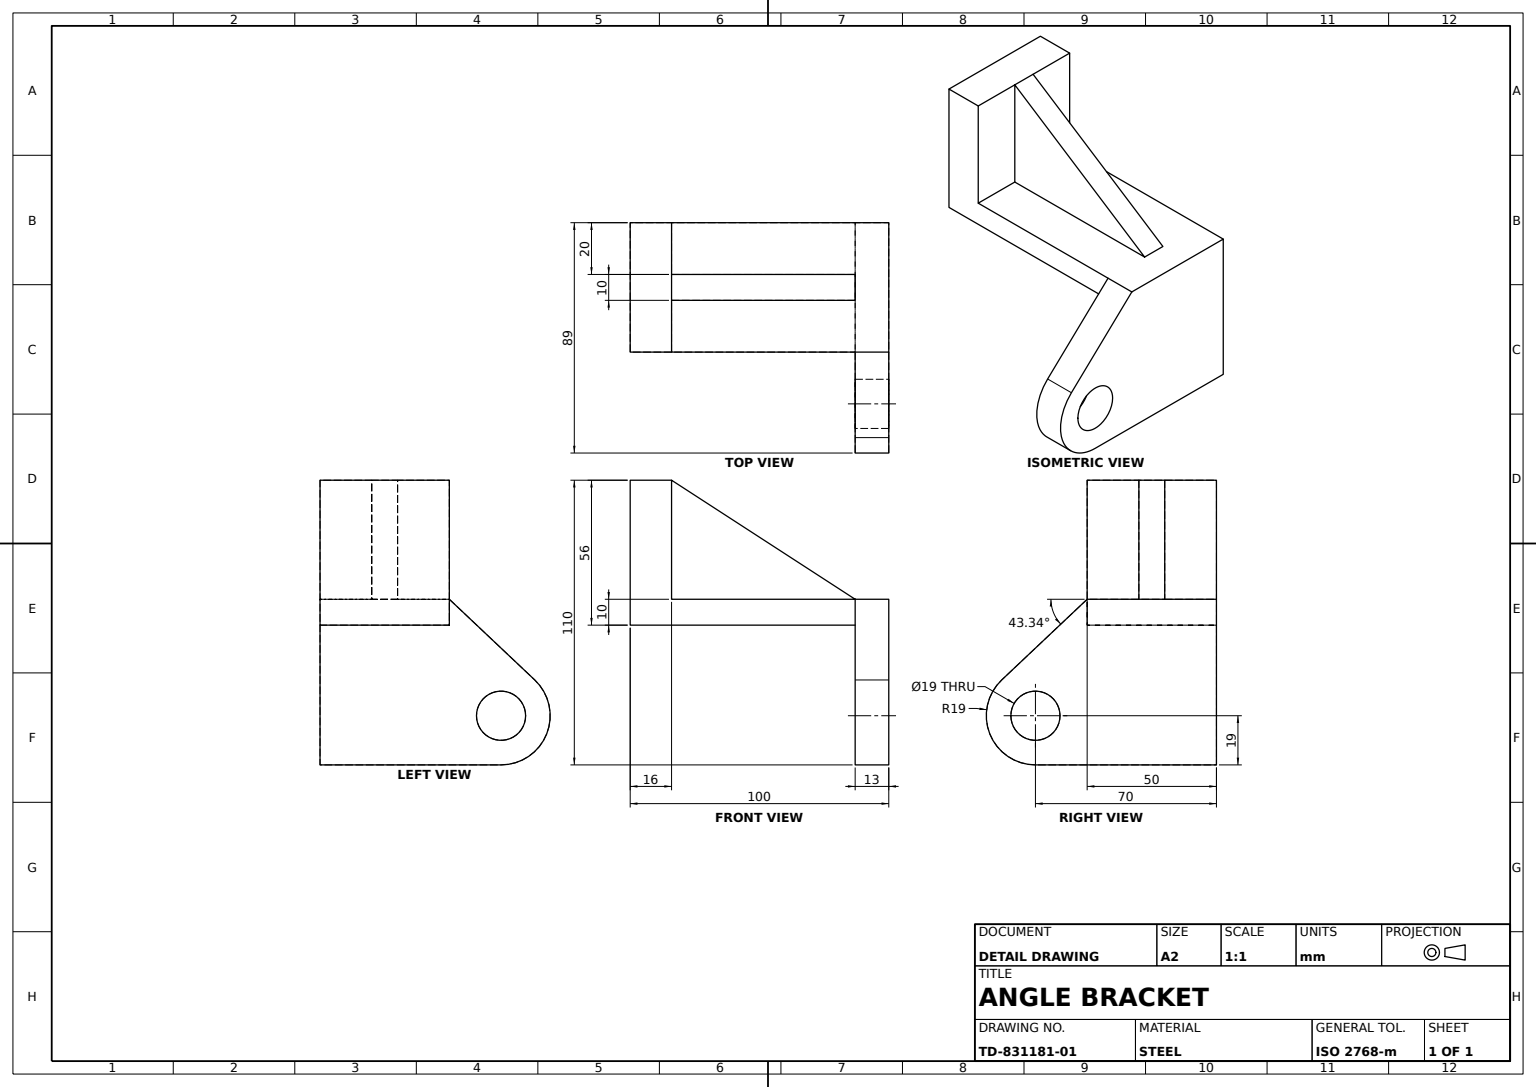
SolidWorks part; units mm, degrees
material "Plain Carbon Steel"
ref_plane "Front Plane" through (0, 0, 0) normal (0, 0, 1) x (1, 0, 0)
ref_plane "Top Plane" through (0, 0, 0) normal (0, 1, 0) x (1, 0, 0)
ref_plane "Right Plane" through (0, 0, 0) normal (1, 0, 0) x (0, 0, -1)
sketch "Base Profile Sketch" plane through (0, 0, 0) normal (0, 0, 1) x (1, 0, 0)
  line L0 (0, 0) -> (16, 0)
  line L1 (16, 0) -> (100, 0)
  line L2 (100, 0) -> (100, 10)
  line L3 (0, 0) -> (0, 56)
  line L4 (0, 56) -> (16, 56)
  line L5 (16, 56) -> (16, 10)
  line L6 (16, 10) -> (100, 10)
  dimension "D1" = 16
  dimension "D2" = 100
  dimension "D3" = 10
  dimension "D4" = 56
extrude "Base Bracket" add sketch "Base Profile Sketch" along normal blind 50
sketch "Pivot Lug Sketch" plane through (100, 0, 0) normal (1, 0, 0) x (0, 0, -1)
  line L0 (0, -54) -> (0, 10)
  line L1 (0, -54) -> (-70, -54)
  line L2 (0, 10) -> (-50, 10)
  line L3 (-50, 10) -> (-83.0407, -21.1819)
  line L4 (0, 0) -> (0, 10) construction
  arc A1 (-83.0407, -21.1819) -> (-70, -54) centre (-70, -35) ccw
  dimension "D1" = 19
  dimension "D2" = 70
  dimension "D3" = 83.0407
extrude "Pivot Lug" add sketch "Pivot Lug Sketch" against normal blind 13
sketch "Pivot Hole Sketch" plane through (100, 0, 0) normal (1, 0, 0) x (0, 0, -1)
  circle A0 centre (-70, -35) radius 9.5
  dimension "D1" = 19
  dimension "D2" = 19
extrude "Pivot Hole Ø19" cut sketch "Pivot Hole Sketch" against normal blind 13
sketch "Gusset Sketch" plane through (0, 0, 50) normal (0, 0, 1) x (1, 0, 0)
  line L0 (16, 56) -> (16, 10)
  line L1 (16, 10) -> (87, 10)
  line L2 (87, 10) -> (16, 56)
extrude "Gusset" add sketch "Gusset Sketch" against normal blind 30
sketch "Gusset Trim Sketch" plane through (0, 0, 50) normal (0, 0, 1) x (1, 0, 0)
  line L0 (16, 56) -> (16, 10)
  line L1 (16, 10) -> (87, 10)
  line L2 (87, 10) -> (16, 56)
extrude "Gusset Trim Cut" cut sketch "Gusset Trim Sketch" against normal blind 20
